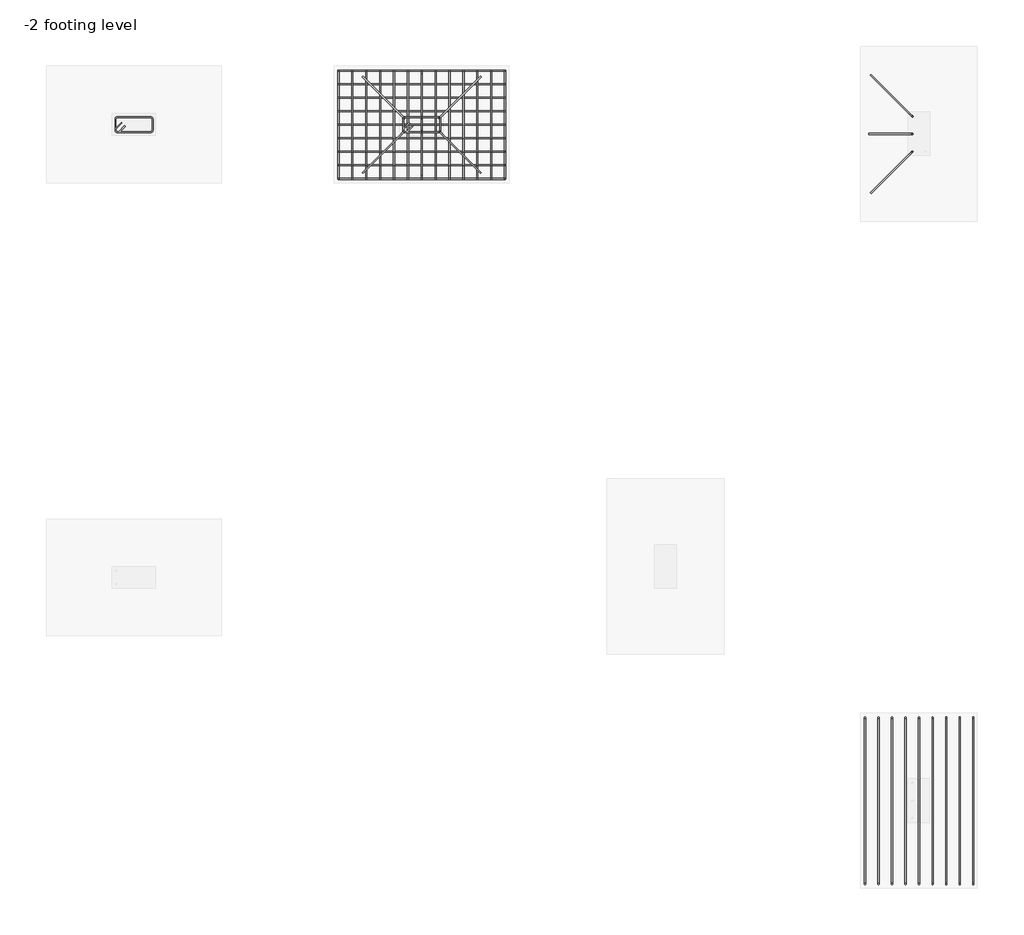
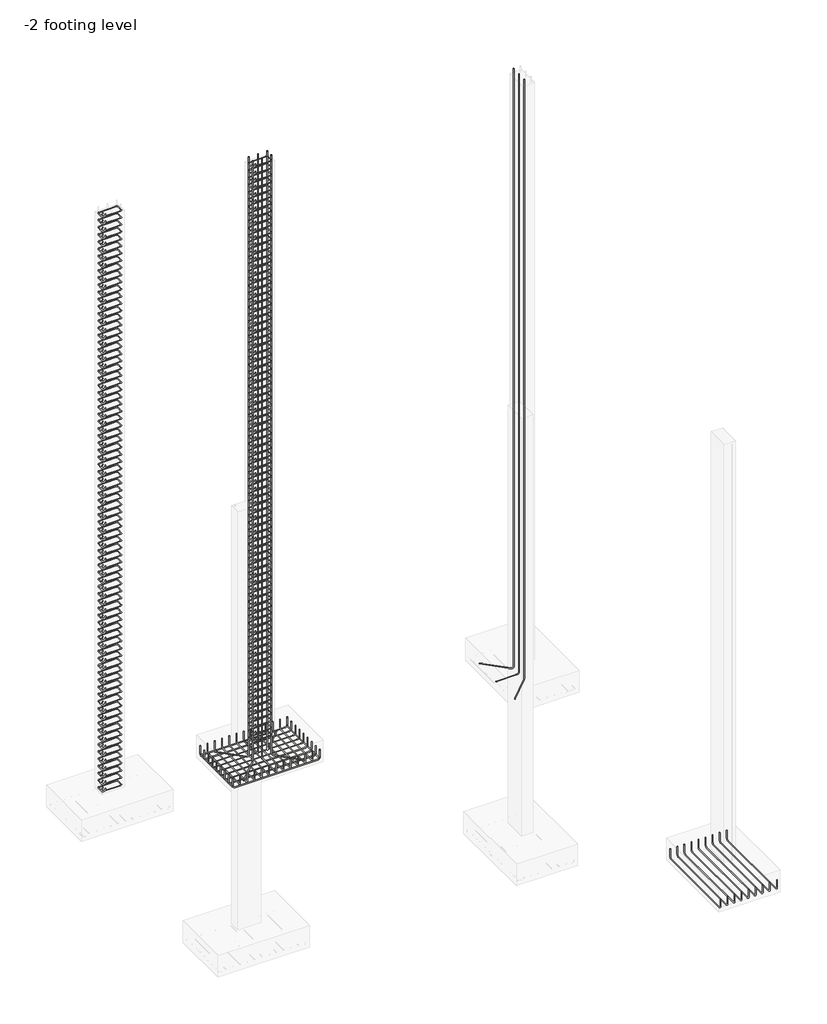
# One storey, part 3 of 9: 14 reinforcing bars.
"""IFC4 building model written with IfcOpenShell, lengths in millimetres."""

from ifc_helpers import new_model, si_unit, point, frame, origin, place, context, project, spatial, polyline, circle_curve, trimmed, segment, composite_curve, source, transform, mapped, element, save
from ifc_brep_helpers import swept_disk

model = new_model("IFC4")

# Units and contexts
model_context = context("Model", 3, world=origin())
ifc_project = project(units=[si_unit("LENGTHUNIT", "METRE", prefix="MILLI")], contexts=[model_context])

# Site, building, storey
site = spatial("IfcSite", under=ifc_project)
building = spatial("IfcBuilding", under=site)
storey = spatial("IfcBuildingStorey", under=building, Name="-2 footing level", Elevation=-1828.8)

# Reinforcing bars
placement = place(None, origin())
reinforcing_bar_shape = source(origin(), model_context, "Body", "SolidModel", [
    swept_disk(composite_curve([segment(polyline([(-4080.5198352, -1961.0445725, -2044.7), (-4080.5198352, -1961.0445725, -2197.1)]), True, "CONTINUOUS"), segment(trimmed(circle_curve(frame((-4124.9698352, -1961.0445725, -2197.1), z_axis=(0.0, 1.0, 0.0), x_axis=(44.44999999999936, 0.0, 0.0)), 44.45), [point((-4080.5198352, -1961.0445725, -2197.1))], [point((-4124.9698352, -1961.0445725, -2241.55))], True, "CARTESIAN"), True, "CONTINUOUS"), segment(polyline([(-4124.9698352, -1961.0445725, -2241.55), (-5775.9698352, -1961.0445725, -2241.55)]), True, "CONTINUOUS"), segment(trimmed(circle_curve(frame((-5775.9698352, -1961.0445725, -2197.1), z_axis=(0.0, 1.0, 0.0), x_axis=(0.0, 0.0, -44.45000000000027)), 44.45), [point((-5775.9698352, -1961.0445725, -2241.55))], [point((-5820.4198352, -1961.0445725, -2197.1))], True, "CARTESIAN"), True, "CONTINUOUS"), segment(polyline([(-5820.4198352, -1961.0445725, -2197.1), (-5820.4198352, -1961.0445725, -2044.7)]), True, "CONTINUOUS")], self_intersect=False), 6.35),
])
element("IfcReinforcingBar", 1, at=placement, inside=storey, context=model_context, shape_type="MappedRepresentation", body=[
    mapped(reinforcing_bar_shape, transform((0.0, 0.0, 0.0), x_axis=(1.0, 0.0, 0.0), y_axis=(0.0, 1.0, 0.0), z_axis=(0.0, 0.0, 1.0))),
    mapped(reinforcing_bar_shape, transform((0.0, -141.2875, 0.0), x_axis=(1.0, 0.0, 0.0), y_axis=(0.0, 1.0, 0.0), z_axis=(0.0, 0.0, 1.0))),
    mapped(reinforcing_bar_shape, transform((0.0, -282.575, 0.0), x_axis=(1.0, 0.0, 0.0), y_axis=(0.0, 1.0, 0.0), z_axis=(0.0, 0.0, 1.0))),
    mapped(reinforcing_bar_shape, transform((0.0, -423.8625, 0.0), x_axis=(1.0, 0.0, 0.0), y_axis=(0.0, 1.0, 0.0), z_axis=(0.0, 0.0, 1.0))),
    mapped(reinforcing_bar_shape, transform((0.0, -565.15, 0.0), x_axis=(1.0, 0.0, 0.0), y_axis=(0.0, 1.0, 0.0), z_axis=(0.0, 0.0, 1.0))),
    mapped(reinforcing_bar_shape, transform((0.0, -706.4375, 0.0), x_axis=(1.0, 0.0, 0.0), y_axis=(0.0, 1.0, 0.0), z_axis=(0.0, 0.0, 1.0))),
    mapped(reinforcing_bar_shape, transform((0.0, -847.725, 0.0), x_axis=(1.0, 0.0, 0.0), y_axis=(0.0, 1.0, 0.0), z_axis=(0.0, 0.0, 1.0))),
    mapped(reinforcing_bar_shape, transform((0.0, -989.0125, 0.0), x_axis=(1.0, 0.0, 0.0), y_axis=(0.0, 1.0, 0.0), z_axis=(0.0, 0.0, 1.0))),
    mapped(reinforcing_bar_shape, transform((0.0, -1130.3, 0.0), x_axis=(1.0, 0.0, 0.0), y_axis=(0.0, 1.0, 0.0), z_axis=(0.0, 0.0, 1.0))),
])
reinforcing_bar_2_shape = source(origin(), model_context, "Body", "SolidModel", [
    swept_disk(composite_curve([segment(polyline([(-5820.4198352, -1961.0445725, -2033.4041416), (-5820.4198352, -1961.0445725, -2185.8041416)]), True, "CONTINUOUS"), segment(trimmed(circle_curve(frame((-5820.4198352, -2005.4945725, -2185.8041416), z_axis=(-1.0, 0.0, 0.0), x_axis=(0.0, 44.450000000000045, 0.0)), 44.45), [point((-5820.4198352, -1961.0445725, -2185.8041416))], [point((-5820.4198352, -2005.4945725, -2230.2541416))], True, "CARTESIAN"), True, "CONTINUOUS"), segment(polyline([(-5820.4198352, -2005.4945725, -2230.2541416), (-5820.4198352, -3046.8945725, -2230.2541416)]), True, "CONTINUOUS"), segment(trimmed(circle_curve(frame((-5820.4198352, -3046.8945725, -2185.8041416), z_axis=(-1.0, 0.0, 0.0), x_axis=(0.0, 0.0, -44.44999999999982)), 44.45), [point((-5820.4198352, -3046.8945725, -2230.2541416))], [point((-5820.4198352, -3091.3445725, -2185.8041416))], True, "CARTESIAN"), True, "CONTINUOUS"), segment(polyline([(-5820.4198352, -3091.3445725, -2185.8041416), (-5820.4198352, -3091.3445725, -2033.4041416)]), True, "CONTINUOUS")], self_intersect=False), 6.35),
])
element("IfcReinforcingBar", 2, at=placement, inside=storey, context=model_context, shape_type="MappedRepresentation", body=[
    mapped(reinforcing_bar_2_shape, transform((0.0, 0.0, 0.0), x_axis=(1.0, 0.0, 0.0), y_axis=(0.0, 1.0, 0.0), z_axis=(0.0, 0.0, 1.0))),
    mapped(reinforcing_bar_2_shape, transform((144.9916667, 0.0, 0.0), x_axis=(1.0, 0.0, 0.0), y_axis=(0.0, 1.0, 0.0), z_axis=(0.0, 0.0, 1.0))),
    mapped(reinforcing_bar_2_shape, transform((289.9833333, 0.0, 0.0), x_axis=(1.0, 0.0, 0.0), y_axis=(0.0, 1.0, 0.0), z_axis=(0.0, 0.0, 1.0))),
    mapped(reinforcing_bar_2_shape, transform((434.975, 0.0, 0.0), x_axis=(1.0, 0.0, 0.0), y_axis=(0.0, 1.0, 0.0), z_axis=(0.0, 0.0, 1.0))),
    mapped(reinforcing_bar_2_shape, transform((579.9666667, 0.0, 0.0), x_axis=(1.0, 0.0, 0.0), y_axis=(0.0, 1.0, 0.0), z_axis=(0.0, 0.0, 1.0))),
    mapped(reinforcing_bar_2_shape, transform((724.9583333, 0.0, 0.0), x_axis=(1.0, 0.0, 0.0), y_axis=(0.0, 1.0, 0.0), z_axis=(0.0, 0.0, 1.0))),
    mapped(reinforcing_bar_2_shape, transform((869.95, 0.0, 0.0), x_axis=(1.0, 0.0, 0.0), y_axis=(0.0, 1.0, 0.0), z_axis=(0.0, 0.0, 1.0))),
    mapped(reinforcing_bar_2_shape, transform((1014.9416667, 0.0, 0.0), x_axis=(1.0, 0.0, 0.0), y_axis=(0.0, 1.0, 0.0), z_axis=(0.0, 0.0, 1.0))),
    mapped(reinforcing_bar_2_shape, transform((1159.9333333, 0.0, 0.0), x_axis=(1.0, 0.0, 0.0), y_axis=(0.0, 1.0, 0.0), z_axis=(0.0, 0.0, 1.0))),
    mapped(reinforcing_bar_2_shape, transform((1304.925, 0.0, 0.0), x_axis=(1.0, 0.0, 0.0), y_axis=(0.0, 1.0, 0.0), z_axis=(0.0, 0.0, 1.0))),
    mapped(reinforcing_bar_2_shape, transform((1449.9166667, 0.0, 0.0), x_axis=(1.0, 0.0, 0.0), y_axis=(0.0, 1.0, 0.0), z_axis=(0.0, 0.0, 1.0))),
    mapped(reinforcing_bar_2_shape, transform((1594.9083333, 0.0, 0.0), x_axis=(1.0, 0.0, 0.0), y_axis=(0.0, 1.0, 0.0), z_axis=(0.0, 0.0, 1.0))),
    mapped(reinforcing_bar_2_shape, transform((1739.9, 0.0, 0.0), x_axis=(1.0, 0.0, 0.0), y_axis=(0.0, 1.0, 0.0), z_axis=(0.0, 0.0, 1.0))),
])
reinforcing_bar_3_shape = source(origin(), model_context, "Body", "SolidModel", [
    swept_disk(composite_curve([segment(polyline([(-321.1911705, -8721.6294723, -2044.7), (-321.1911705, -8721.6294723, -2197.1)]), True, "CONTINUOUS"), segment(trimmed(circle_curve(frame((-321.1911705, -8766.0794723, -2197.1), z_axis=(-1.0, 0.0, 0.0), x_axis=(0.0, 44.45000000000073, 0.0)), 44.45), [point((-321.1911705, -8721.6294723, -2197.1))], [point((-321.1911705, -8766.0794723, -2241.55))], True, "CARTESIAN"), True, "CONTINUOUS"), segment(polyline([(-321.1911705, -8766.0794723, -2241.55), (-321.1911705, -10417.0794723, -2241.55)]), True, "CONTINUOUS"), segment(trimmed(circle_curve(frame((-321.1911705, -10417.0794723, -2197.1), z_axis=(-1.0, 0.0, 0.0), x_axis=(0.0, 0.0, -44.45000000000027)), 44.45), [point((-321.1911705, -10417.0794723, -2241.55))], [point((-321.1911705, -10461.5294723, -2197.1))], True, "CARTESIAN"), True, "CONTINUOUS"), segment(polyline([(-321.1911705, -10461.5294723, -2197.1), (-321.1911705, -10461.5294723, -2044.7)]), True, "CONTINUOUS")], self_intersect=False), 6.35),
])
element("IfcReinforcingBar", 3, at=placement, inside=storey, context=model_context, shape_type="MappedRepresentation", body=[
    mapped(reinforcing_bar_3_shape, transform((0.0, 0.0, 0.0), x_axis=(1.0, 0.0, 0.0), y_axis=(0.0, 1.0, 0.0), z_axis=(0.0, 0.0, 1.0))),
    mapped(reinforcing_bar_3_shape, transform((141.2875, 0.0, 0.0), x_axis=(1.0, 0.0, 0.0), y_axis=(0.0, 1.0, 0.0), z_axis=(0.0, 0.0, 1.0))),
    mapped(reinforcing_bar_3_shape, transform((282.575, 0.0, 0.0), x_axis=(1.0, 0.0, 0.0), y_axis=(0.0, 1.0, 0.0), z_axis=(0.0, 0.0, 1.0))),
    mapped(reinforcing_bar_3_shape, transform((423.8625, 0.0, 0.0), x_axis=(1.0, 0.0, 0.0), y_axis=(0.0, 1.0, 0.0), z_axis=(0.0, 0.0, 1.0))),
    mapped(reinforcing_bar_3_shape, transform((565.15, 0.0, 0.0), x_axis=(1.0, 0.0, 0.0), y_axis=(0.0, 1.0, 0.0), z_axis=(0.0, 0.0, 1.0))),
    mapped(reinforcing_bar_3_shape, transform((706.4375, 0.0, 0.0), x_axis=(1.0, 0.0, 0.0), y_axis=(0.0, 1.0, 0.0), z_axis=(0.0, 0.0, 1.0))),
    mapped(reinforcing_bar_3_shape, transform((847.725, 0.0, 0.0), x_axis=(1.0, 0.0, 0.0), y_axis=(0.0, 1.0, 0.0), z_axis=(0.0, 0.0, 1.0))),
    mapped(reinforcing_bar_3_shape, transform((989.0125, 0.0, 0.0), x_axis=(1.0, 0.0, 0.0), y_axis=(0.0, 1.0, 0.0), z_axis=(0.0, 0.0, 1.0))),
    mapped(reinforcing_bar_3_shape, transform((1130.3, 0.0, 0.0), x_axis=(1.0, 0.0, 0.0), y_axis=(0.0, 1.0, 0.0), z_axis=(0.0, 0.0, 1.0))),
])
element("IfcReinforcingBar", 4, at=placement, inside=storey, context=model_context, shape_type="SolidModel", body=[
    swept_disk(composite_curve([segment(polyline([(-259.3446547, -3240.9386149, -2212.9582082), (142.6779331, -2838.9160271, -2212.9582082)]), True, "CONTINUOUS"), segment(trimmed(circle_curve(frame((142.6779331, -2838.9160271, -2168.5082082), z_axis=(0.7071067811865501, -0.7071067811865449, 0.0), x_axis=(0.0, 0.0, -44.45000000000027)), 44.45), [point((142.6779331, -2838.9160271, -2212.9582082))], [point((174.1088295, -2807.4851307, -2168.5082082))], True, "CARTESIAN"), True, "CONTINUOUS"), segment(polyline([(174.1088295, -2807.4851307, -2168.5082082), (174.1088295, -2807.4851307, 10477.5)]), True, "CONTINUOUS")], self_intersect=False), 6.35),
])
element("IfcReinforcingBar", 5, at=placement, inside=storey, context=model_context, shape_type="SolidModel", body=[
    swept_disk(composite_curve([segment(polyline([(-259.3446547, -2005.7316465, -2212.9582082), (142.6779331, -2407.7542342, -2212.9582082)]), True, "CONTINUOUS"), segment(trimmed(circle_curve(frame((142.6779331, -2407.7542342, -2168.5082082), z_axis=(-0.7071067811865501, -0.7071067811865449, 0.0), x_axis=(0.0, 0.0, -44.45000000000027)), 44.45), [point((142.6779331, -2407.7542342, -2212.9582082))], [point((174.1088295, -2439.1851307, -2168.5082082))], True, "CARTESIAN"), True, "CONTINUOUS"), segment(polyline([(174.1088295, -2439.1851307, -2168.5082082), (174.1088295, -2439.1851307, 10477.5)]), True, "CONTINUOUS")], self_intersect=False), 6.35),
])
element("IfcReinforcingBar", 6, at=placement, inside=storey, context=model_context, shape_type="SolidModel", body=[
    swept_disk(composite_curve([segment(polyline([(-283.0911705, -2623.3351307, -2212.9582082), (129.6588295, -2623.3351307, -2212.9582082)]), True, "CONTINUOUS"), segment(trimmed(circle_curve(frame((129.6588295, -2623.3351307, -2168.5082082), z_axis=(0.0, -1.0, 0.0), x_axis=(0.0, 0.0, -44.45000000000027)), 44.45), [point((129.6588295, -2623.3351307, -2212.9582082))], [point((174.1088295, -2623.3351307, -2168.5082082))], True, "CARTESIAN"), True, "CONTINUOUS"), segment(polyline([(174.1088295, -2623.3351307, -2168.5082082), (174.1088295, -2623.3351307, 10477.5)]), True, "CONTINUOUS")], self_intersect=False), 6.35),
])
reinforcing_bar_4_shape = source(origin(), model_context, "Body", "SolidModel", [
    swept_disk(composite_curve([segment(polyline([(-8086.1371138, -2508.2533327, -1794.0734375), (-8143.0013108, -2565.1175298, -1794.0734375)]), True, "CONTINUOUS"), segment(trimmed(circle_curve(frame((-8126.1633306, -2581.95551, -1794.0734375), z_axis=(0.0, 0.0, 1.0), x_axis=(-16.837980199999947, 16.837980199999947, 0.0)), 23.8125), [point((-8143.0013108, -2565.1175298, -1794.0734375))], [point((-8126.1633306, -2605.76801, -1794.0734375))], True, "CARTESIAN"), True, "CONTINUOUS"), segment(polyline([(-8126.1633306, -2605.76801, -1794.0734375), (-7786.0414556, -2605.76801, -1794.0734375)]), True, "CONTINUOUS"), segment(trimmed(circle_curve(frame((-7786.0414556, -2581.95551, -1794.0734375), z_axis=(0.0, 0.0, 1.0), x_axis=(0.0, -23.8125, 0.0)), 23.8125), [point((-7786.0414556, -2605.76801, -1794.0734375))], [point((-7762.2289556, -2581.95551, -1794.0734375))], True, "CARTESIAN"), True, "CONTINUOUS"), segment(polyline([(-7762.2289556, -2581.95551, -1794.0734375), (-7762.2289556, -2470.433635, -1794.0734375)]), True, "CONTINUOUS"), segment(trimmed(circle_curve(frame((-7786.0342742, -2470.433635, -1794.658215), z_axis=(-0.024557586497356516, 0.0, 0.9996984169965585), x_axis=(23.805318600000646, 0.0, 0.5847774999999729)), 23.8125), [point((-7762.2289556, -2470.433635, -1794.0734375))], [point((-7786.0342742, -2446.621135, -1794.658215))], True, "CARTESIAN"), True, "CONTINUOUS"), segment(polyline([(-7786.0342742, -2446.621135, -1794.658215), (-8126.170512, -2446.621135, -1803.01366)]), True, "CONTINUOUS"), segment(trimmed(circle_curve(frame((-8126.170512, -2470.433635, -1803.01366), z_axis=(-0.024557586497356516, 0.0, 0.9996984169965585), x_axis=(0.0, 23.8125, 0.0)), 23.8125), [point((-8126.170512, -2446.621135, -1803.01366))], [point((-8149.9758306, -2470.433635, -1803.5984375))], True, "CARTESIAN"), True, "CONTINUOUS"), segment(polyline([(-8149.9758306, -2470.433635, -1803.5984375), (-8149.9758306, -2581.95551, -1803.5984375)]), True, "CONTINUOUS"), segment(trimmed(circle_curve(frame((-8126.1633306, -2581.95551, -1803.5984375), z_axis=(0.0, 0.0, 1.0), x_axis=(-23.8125, 0.0, 0.0)), 23.8125), [point((-8149.9758306, -2581.95551, -1803.5984375))], [point((-8109.3253504, -2598.7934902, -1803.5984375))], True, "CARTESIAN"), True, "CONTINUOUS"), segment(polyline([(-8109.3253504, -2598.7934902, -1803.5984375), (-8052.4611533, -2541.9292932, -1803.5984375)]), True, "CONTINUOUS")], self_intersect=False), 4.7625),
])
element("IfcReinforcingBar", 7, at=placement, inside=storey, context=model_context, shape_type="MappedRepresentation", body=[
    mapped(reinforcing_bar_4_shape, transform((0.0, 0.0, 0.0), x_axis=(1.0, 0.0, 0.0), y_axis=(0.0, 1.0, 0.0), z_axis=(0.0, 0.0, 1.0))),
    mapped(reinforcing_bar_4_shape, transform((0.0, 0.0, 151.9063867), x_axis=(1.0, 0.0, 0.0), y_axis=(0.0, 1.0, 0.0), z_axis=(0.0, 0.0, 1.0))),
    mapped(reinforcing_bar_4_shape, transform((0.0, 0.0, 303.8127734), x_axis=(1.0, 0.0, 0.0), y_axis=(0.0, 1.0, 0.0), z_axis=(0.0, 0.0, 1.0))),
    mapped(reinforcing_bar_4_shape, transform((0.0, 0.0, 455.7191602), x_axis=(1.0, 0.0, 0.0), y_axis=(0.0, 1.0, 0.0), z_axis=(0.0, 0.0, 1.0))),
    mapped(reinforcing_bar_4_shape, transform((0.0, 0.0, 607.6255469), x_axis=(1.0, 0.0, 0.0), y_axis=(0.0, 1.0, 0.0), z_axis=(0.0, 0.0, 1.0))),
    mapped(reinforcing_bar_4_shape, transform((0.0, 0.0, 759.5319336), x_axis=(1.0, 0.0, 0.0), y_axis=(0.0, 1.0, 0.0), z_axis=(0.0, 0.0, 1.0))),
    mapped(reinforcing_bar_4_shape, transform((0.0, 0.0, 911.4383203), x_axis=(1.0, 0.0, 0.0), y_axis=(0.0, 1.0, 0.0), z_axis=(0.0, 0.0, 1.0))),
    mapped(reinforcing_bar_4_shape, transform((0.0, 0.0, 1063.344707), x_axis=(1.0, 0.0, 0.0), y_axis=(0.0, 1.0, 0.0), z_axis=(0.0, 0.0, 1.0))),
    mapped(reinforcing_bar_4_shape, transform((0.0, 0.0, 1215.2510937), x_axis=(1.0, 0.0, 0.0), y_axis=(0.0, 1.0, 0.0), z_axis=(0.0, 0.0, 1.0))),
    mapped(reinforcing_bar_4_shape, transform((0.0, 0.0, 1367.1574805), x_axis=(1.0, 0.0, 0.0), y_axis=(0.0, 1.0, 0.0), z_axis=(0.0, 0.0, 1.0))),
    mapped(reinforcing_bar_4_shape, transform((0.0, 0.0, 1519.0638672), x_axis=(1.0, 0.0, 0.0), y_axis=(0.0, 1.0, 0.0), z_axis=(0.0, 0.0, 1.0))),
    mapped(reinforcing_bar_4_shape, transform((0.0, 0.0, 1670.9702539), x_axis=(1.0, 0.0, 0.0), y_axis=(0.0, 1.0, 0.0), z_axis=(0.0, 0.0, 1.0))),
    mapped(reinforcing_bar_4_shape, transform((0.0, 0.0, 1822.8766406), x_axis=(1.0, 0.0, 0.0), y_axis=(0.0, 1.0, 0.0), z_axis=(0.0, 0.0, 1.0))),
    mapped(reinforcing_bar_4_shape, transform((0.0, 0.0, 1974.7830273), x_axis=(1.0, 0.0, 0.0), y_axis=(0.0, 1.0, 0.0), z_axis=(0.0, 0.0, 1.0))),
    mapped(reinforcing_bar_4_shape, transform((0.0, 0.0, 2126.6894141), x_axis=(1.0, 0.0, 0.0), y_axis=(0.0, 1.0, 0.0), z_axis=(0.0, 0.0, 1.0))),
    mapped(reinforcing_bar_4_shape, transform((0.0, 0.0, 2278.5958008), x_axis=(1.0, 0.0, 0.0), y_axis=(0.0, 1.0, 0.0), z_axis=(0.0, 0.0, 1.0))),
    mapped(reinforcing_bar_4_shape, transform((0.0, 0.0, 2430.5021875), x_axis=(1.0, 0.0, 0.0), y_axis=(0.0, 1.0, 0.0), z_axis=(0.0, 0.0, 1.0))),
    mapped(reinforcing_bar_4_shape, transform((0.0, 0.0, 2582.4085742), x_axis=(1.0, 0.0, 0.0), y_axis=(0.0, 1.0, 0.0), z_axis=(0.0, 0.0, 1.0))),
    mapped(reinforcing_bar_4_shape, transform((0.0, 0.0, 2734.3149609), x_axis=(1.0, 0.0, 0.0), y_axis=(0.0, 1.0, 0.0), z_axis=(0.0, 0.0, 1.0))),
    mapped(reinforcing_bar_4_shape, transform((0.0, 0.0, 2886.2213477), x_axis=(1.0, 0.0, 0.0), y_axis=(0.0, 1.0, 0.0), z_axis=(0.0, 0.0, 1.0))),
    mapped(reinforcing_bar_4_shape, transform((0.0, 0.0, 3038.1277344), x_axis=(1.0, 0.0, 0.0), y_axis=(0.0, 1.0, 0.0), z_axis=(0.0, 0.0, 1.0))),
    mapped(reinforcing_bar_4_shape, transform((0.0, 0.0, 3190.0341211), x_axis=(1.0, 0.0, 0.0), y_axis=(0.0, 1.0, 0.0), z_axis=(0.0, 0.0, 1.0))),
    mapped(reinforcing_bar_4_shape, transform((0.0, 0.0, 3341.9405078), x_axis=(1.0, 0.0, 0.0), y_axis=(0.0, 1.0, 0.0), z_axis=(0.0, 0.0, 1.0))),
    mapped(reinforcing_bar_4_shape, transform((0.0, 0.0, 3493.8468945), x_axis=(1.0, 0.0, 0.0), y_axis=(0.0, 1.0, 0.0), z_axis=(0.0, 0.0, 1.0))),
    mapped(reinforcing_bar_4_shape, transform((0.0, 0.0, 3645.7532812), x_axis=(1.0, 0.0, 0.0), y_axis=(0.0, 1.0, 0.0), z_axis=(0.0, 0.0, 1.0))),
    mapped(reinforcing_bar_4_shape, transform((0.0, 0.0, 3797.659668), x_axis=(1.0, 0.0, 0.0), y_axis=(0.0, 1.0, 0.0), z_axis=(0.0, 0.0, 1.0))),
    mapped(reinforcing_bar_4_shape, transform((0.0, 0.0, 3949.5660547), x_axis=(1.0, 0.0, 0.0), y_axis=(0.0, 1.0, 0.0), z_axis=(0.0, 0.0, 1.0))),
    mapped(reinforcing_bar_4_shape, transform((0.0, 0.0, 4101.4724414), x_axis=(1.0, 0.0, 0.0), y_axis=(0.0, 1.0, 0.0), z_axis=(0.0, 0.0, 1.0))),
    mapped(reinforcing_bar_4_shape, transform((0.0, 0.0, 4253.3788281), x_axis=(1.0, 0.0, 0.0), y_axis=(0.0, 1.0, 0.0), z_axis=(0.0, 0.0, 1.0))),
    mapped(reinforcing_bar_4_shape, transform((0.0, 0.0, 4405.2852148), x_axis=(1.0, 0.0, 0.0), y_axis=(0.0, 1.0, 0.0), z_axis=(0.0, 0.0, 1.0))),
    mapped(reinforcing_bar_4_shape, transform((0.0, 0.0, 4557.1916016), x_axis=(1.0, 0.0, 0.0), y_axis=(0.0, 1.0, 0.0), z_axis=(0.0, 0.0, 1.0))),
    mapped(reinforcing_bar_4_shape, transform((0.0, 0.0, 4709.0979883), x_axis=(1.0, 0.0, 0.0), y_axis=(0.0, 1.0, 0.0), z_axis=(0.0, 0.0, 1.0))),
    mapped(reinforcing_bar_4_shape, transform((0.0, 0.0, 4861.004375), x_axis=(1.0, 0.0, 0.0), y_axis=(0.0, 1.0, 0.0), z_axis=(0.0, 0.0, 1.0))),
    mapped(reinforcing_bar_4_shape, transform((0.0, 0.0, 5012.9107617), x_axis=(1.0, 0.0, 0.0), y_axis=(0.0, 1.0, 0.0), z_axis=(0.0, 0.0, 1.0))),
    mapped(reinforcing_bar_4_shape, transform((0.0, 0.0, 5164.8171484), x_axis=(1.0, 0.0, 0.0), y_axis=(0.0, 1.0, 0.0), z_axis=(0.0, 0.0, 1.0))),
    mapped(reinforcing_bar_4_shape, transform((0.0, 0.0, 5316.7235352), x_axis=(1.0, 0.0, 0.0), y_axis=(0.0, 1.0, 0.0), z_axis=(0.0, 0.0, 1.0))),
    mapped(reinforcing_bar_4_shape, transform((0.0, 0.0, 5468.6299219), x_axis=(1.0, 0.0, 0.0), y_axis=(0.0, 1.0, 0.0), z_axis=(0.0, 0.0, 1.0))),
    mapped(reinforcing_bar_4_shape, transform((0.0, 0.0, 5620.5363086), x_axis=(1.0, 0.0, 0.0), y_axis=(0.0, 1.0, 0.0), z_axis=(0.0, 0.0, 1.0))),
    mapped(reinforcing_bar_4_shape, transform((0.0, 0.0, 5772.4426953), x_axis=(1.0, 0.0, 0.0), y_axis=(0.0, 1.0, 0.0), z_axis=(0.0, 0.0, 1.0))),
    mapped(reinforcing_bar_4_shape, transform((0.0, 0.0, 5924.349082), x_axis=(1.0, 0.0, 0.0), y_axis=(0.0, 1.0, 0.0), z_axis=(0.0, 0.0, 1.0))),
    mapped(reinforcing_bar_4_shape, transform((0.0, 0.0, 6076.2554687), x_axis=(1.0, 0.0, 0.0), y_axis=(0.0, 1.0, 0.0), z_axis=(0.0, 0.0, 1.0))),
    mapped(reinforcing_bar_4_shape, transform((0.0, 0.0, 6228.1618555), x_axis=(1.0, 0.0, 0.0), y_axis=(0.0, 1.0, 0.0), z_axis=(0.0, 0.0, 1.0))),
    mapped(reinforcing_bar_4_shape, transform((0.0, 0.0, 6380.0682422), x_axis=(1.0, 0.0, 0.0), y_axis=(0.0, 1.0, 0.0), z_axis=(0.0, 0.0, 1.0))),
    mapped(reinforcing_bar_4_shape, transform((0.0, 0.0, 6531.9746289), x_axis=(1.0, 0.0, 0.0), y_axis=(0.0, 1.0, 0.0), z_axis=(0.0, 0.0, 1.0))),
    mapped(reinforcing_bar_4_shape, transform((0.0, 0.0, 6683.8810156), x_axis=(1.0, 0.0, 0.0), y_axis=(0.0, 1.0, 0.0), z_axis=(0.0, 0.0, 1.0))),
    mapped(reinforcing_bar_4_shape, transform((0.0, 0.0, 6835.7874023), x_axis=(1.0, 0.0, 0.0), y_axis=(0.0, 1.0, 0.0), z_axis=(0.0, 0.0, 1.0))),
    mapped(reinforcing_bar_4_shape, transform((0.0, 0.0, 6987.6937891), x_axis=(1.0, 0.0, 0.0), y_axis=(0.0, 1.0, 0.0), z_axis=(0.0, 0.0, 1.0))),
    mapped(reinforcing_bar_4_shape, transform((0.0, 0.0, 7139.6001758), x_axis=(1.0, 0.0, 0.0), y_axis=(0.0, 1.0, 0.0), z_axis=(0.0, 0.0, 1.0))),
    mapped(reinforcing_bar_4_shape, transform((0.0, 0.0, 7291.5065625), x_axis=(1.0, 0.0, 0.0), y_axis=(0.0, 1.0, 0.0), z_axis=(0.0, 0.0, 1.0))),
    mapped(reinforcing_bar_4_shape, transform((0.0, 0.0, 7443.4129492), x_axis=(1.0, 0.0, 0.0), y_axis=(0.0, 1.0, 0.0), z_axis=(0.0, 0.0, 1.0))),
    mapped(reinforcing_bar_4_shape, transform((0.0, 0.0, 7595.3193359), x_axis=(1.0, 0.0, 0.0), y_axis=(0.0, 1.0, 0.0), z_axis=(0.0, 0.0, 1.0))),
    mapped(reinforcing_bar_4_shape, transform((0.0, 0.0, 7747.2257227), x_axis=(1.0, 0.0, 0.0), y_axis=(0.0, 1.0, 0.0), z_axis=(0.0, 0.0, 1.0))),
    mapped(reinforcing_bar_4_shape, transform((0.0, 0.0, 7899.1321094), x_axis=(1.0, 0.0, 0.0), y_axis=(0.0, 1.0, 0.0), z_axis=(0.0, 0.0, 1.0))),
    mapped(reinforcing_bar_4_shape, transform((0.0, 0.0, 8051.0384961), x_axis=(1.0, 0.0, 0.0), y_axis=(0.0, 1.0, 0.0), z_axis=(0.0, 0.0, 1.0))),
    mapped(reinforcing_bar_4_shape, transform((0.0, 0.0, 8202.9448828), x_axis=(1.0, 0.0, 0.0), y_axis=(0.0, 1.0, 0.0), z_axis=(0.0, 0.0, 1.0))),
    mapped(reinforcing_bar_4_shape, transform((0.0, 0.0, 8354.8512695), x_axis=(1.0, 0.0, 0.0), y_axis=(0.0, 1.0, 0.0), z_axis=(0.0, 0.0, 1.0))),
    mapped(reinforcing_bar_4_shape, transform((0.0, 0.0, 8506.7576562), x_axis=(1.0, 0.0, 0.0), y_axis=(0.0, 1.0, 0.0), z_axis=(0.0, 0.0, 1.0))),
    mapped(reinforcing_bar_4_shape, transform((0.0, 0.0, 8658.664043), x_axis=(1.0, 0.0, 0.0), y_axis=(0.0, 1.0, 0.0), z_axis=(0.0, 0.0, 1.0))),
    mapped(reinforcing_bar_4_shape, transform((0.0, 0.0, 8810.5704297), x_axis=(1.0, 0.0, 0.0), y_axis=(0.0, 1.0, 0.0), z_axis=(0.0, 0.0, 1.0))),
    mapped(reinforcing_bar_4_shape, transform((0.0, 0.0, 8962.4768164), x_axis=(1.0, 0.0, 0.0), y_axis=(0.0, 1.0, 0.0), z_axis=(0.0, 0.0, 1.0))),
    mapped(reinforcing_bar_4_shape, transform((0.0, 0.0, 9114.3832031), x_axis=(1.0, 0.0, 0.0), y_axis=(0.0, 1.0, 0.0), z_axis=(0.0, 0.0, 1.0))),
    mapped(reinforcing_bar_4_shape, transform((0.0, 0.0, 9266.2895898), x_axis=(1.0, 0.0, 0.0), y_axis=(0.0, 1.0, 0.0), z_axis=(0.0, 0.0, 1.0))),
    mapped(reinforcing_bar_4_shape, transform((0.0, 0.0, 9418.1959766), x_axis=(1.0, 0.0, 0.0), y_axis=(0.0, 1.0, 0.0), z_axis=(0.0, 0.0, 1.0))),
    mapped(reinforcing_bar_4_shape, transform((0.0, 0.0, 9570.1023633), x_axis=(1.0, 0.0, 0.0), y_axis=(0.0, 1.0, 0.0), z_axis=(0.0, 0.0, 1.0))),
    mapped(reinforcing_bar_4_shape, transform((0.0, 0.0, 9722.00875), x_axis=(1.0, 0.0, 0.0), y_axis=(0.0, 1.0, 0.0), z_axis=(0.0, 0.0, 1.0))),
    mapped(reinforcing_bar_4_shape, transform((0.0, 0.0, 9873.9151367), x_axis=(1.0, 0.0, 0.0), y_axis=(0.0, 1.0, 0.0), z_axis=(0.0, 0.0, 1.0))),
    mapped(reinforcing_bar_4_shape, transform((0.0, 0.0, 10025.8215234), x_axis=(1.0, 0.0, 0.0), y_axis=(0.0, 1.0, 0.0), z_axis=(0.0, 0.0, 1.0))),
    mapped(reinforcing_bar_4_shape, transform((0.0, 0.0, 10177.7279102), x_axis=(1.0, 0.0, 0.0), y_axis=(0.0, 1.0, 0.0), z_axis=(0.0, 0.0, 1.0))),
    mapped(reinforcing_bar_4_shape, transform((0.0, 0.0, 10329.6342969), x_axis=(1.0, 0.0, 0.0), y_axis=(0.0, 1.0, 0.0), z_axis=(0.0, 0.0, 1.0))),
    mapped(reinforcing_bar_4_shape, transform((0.0, 0.0, 10481.5406836), x_axis=(1.0, 0.0, 0.0), y_axis=(0.0, 1.0, 0.0), z_axis=(0.0, 0.0, 1.0))),
    mapped(reinforcing_bar_4_shape, transform((0.0, 0.0, 10633.4470703), x_axis=(1.0, 0.0, 0.0), y_axis=(0.0, 1.0, 0.0), z_axis=(0.0, 0.0, 1.0))),
    mapped(reinforcing_bar_4_shape, transform((0.0, 0.0, 10785.353457), x_axis=(1.0, 0.0, 0.0), y_axis=(0.0, 1.0, 0.0), z_axis=(0.0, 0.0, 1.0))),
    mapped(reinforcing_bar_4_shape, transform((0.0, 0.0, 10937.2598437), x_axis=(1.0, 0.0, 0.0), y_axis=(0.0, 1.0, 0.0), z_axis=(0.0, 0.0, 1.0))),
    mapped(reinforcing_bar_4_shape, transform((0.0, 0.0, 11089.1662305), x_axis=(1.0, 0.0, 0.0), y_axis=(0.0, 1.0, 0.0), z_axis=(0.0, 0.0, 1.0))),
    mapped(reinforcing_bar_4_shape, transform((0.0, 0.0, 11241.0726172), x_axis=(1.0, 0.0, 0.0), y_axis=(0.0, 1.0, 0.0), z_axis=(0.0, 0.0, 1.0))),
    mapped(reinforcing_bar_4_shape, transform((0.0, 0.0, 11392.9790039), x_axis=(1.0, 0.0, 0.0), y_axis=(0.0, 1.0, 0.0), z_axis=(0.0, 0.0, 1.0))),
    mapped(reinforcing_bar_4_shape, transform((0.0, 0.0, 11544.8853906), x_axis=(1.0, 0.0, 0.0), y_axis=(0.0, 1.0, 0.0), z_axis=(0.0, 0.0, 1.0))),
    mapped(reinforcing_bar_4_shape, transform((0.0, 0.0, 11696.7917773), x_axis=(1.0, 0.0, 0.0), y_axis=(0.0, 1.0, 0.0), z_axis=(0.0, 0.0, 1.0))),
    mapped(reinforcing_bar_4_shape, transform((0.0, 0.0, 11848.6981641), x_axis=(1.0, 0.0, 0.0), y_axis=(0.0, 1.0, 0.0), z_axis=(0.0, 0.0, 1.0))),
    mapped(reinforcing_bar_4_shape, transform((0.0, 0.0, 12000.6045508), x_axis=(1.0, 0.0, 0.0), y_axis=(0.0, 1.0, 0.0), z_axis=(0.0, 0.0, 1.0))),
    mapped(reinforcing_bar_4_shape, transform((0.0, 0.0, 12152.5109375), x_axis=(1.0, 0.0, 0.0), y_axis=(0.0, 1.0, 0.0), z_axis=(0.0, 0.0, 1.0))),
])
element("IfcReinforcingBar", 8, at=placement, inside=storey, context=model_context, shape_type="SolidModel", body=[
    swept_disk(composite_curve([segment(polyline([(-5568.6755659, -2022.8910883, -2212.9582082), (-5166.6529781, -2424.9136761, -2212.9582082)]), True, "CONTINUOUS"), segment(trimmed(circle_curve(frame((-5166.6529781, -2424.9136761, -2168.5082082), z_axis=(-0.7071067811865455, -0.7071067811865496, 0.0), x_axis=(0.0, 0.0, -44.45000000000027)), 44.45), [point((-5166.6529781, -2424.9136761, -2212.9582082))], [point((-5135.2220817, -2456.3445725, -2168.5082082))], True, "CARTESIAN"), True, "CONTINUOUS"), segment(polyline([(-5135.2220817, -2456.3445725, -2168.5082082), (-5135.2220817, -2456.3445725, 10477.5)]), True, "CONTINUOUS")], self_intersect=False), 6.35),
])
element("IfcReinforcingBar", 9, at=placement, inside=storey, context=model_context, shape_type="SolidModel", body=[
    swept_disk(composite_curve([segment(polyline([(-5568.6755659, -3029.4980567, -2212.9582082), (-5166.6529781, -2627.4754689, -2212.9582082)]), True, "CONTINUOUS"), segment(trimmed(circle_curve(frame((-5166.6529781, -2627.4754689, -2168.5082082), z_axis=(0.707106781186541, -0.707106781186554, 0.0), x_axis=(0.0, 0.0, -44.45000000000027)), 44.45), [point((-5166.6529781, -2627.4754689, -2212.9582082))], [point((-5135.2220817, -2596.0445725, -2168.5082082))], True, "CARTESIAN"), True, "CONTINUOUS"), segment(polyline([(-5135.2220817, -2596.0445725, -2168.5082082), (-5135.2220817, -2596.0445725, 10477.5)]), True, "CONTINUOUS")], self_intersect=False), 6.35),
])
element("IfcReinforcingBar", 10, at=placement, inside=storey, context=model_context, shape_type="SolidModel", body=[
    swept_disk(composite_curve([segment(polyline([(-4333.4685975, -2022.8910883, -2212.9582082), (-4735.4911853, -2424.9136761, -2212.9582082)]), True, "CONTINUOUS"), segment(trimmed(circle_curve(frame((-4735.4911853, -2424.9136761, -2168.5082082), z_axis=(-0.7071067811865444, 0.7071067811865507, 0.0), x_axis=(0.0, 0.0, -44.45000000000027)), 44.45), [point((-4735.4911853, -2424.9136761, -2212.9582082))], [point((-4766.9220817, -2456.3445725, -2168.5082082))], True, "CARTESIAN"), True, "CONTINUOUS"), segment(polyline([(-4766.9220817, -2456.3445725, -2168.5082082), (-4766.9220817, -2456.3445725, 10477.5)]), True, "CONTINUOUS")], self_intersect=False), 6.35),
])
element("IfcReinforcingBar", 11, at=placement, inside=storey, context=model_context, shape_type="SolidModel", body=[
    swept_disk(composite_curve([segment(polyline([(-4333.4685975, -3029.4980567, -2212.9582082), (-4735.4911853, -2627.4754689, -2212.9582082)]), True, "CONTINUOUS"), segment(trimmed(circle_curve(frame((-4735.4911853, -2627.4754689, -2168.5082082), z_axis=(0.7071067811865421, 0.7071067811865529, 0.0), x_axis=(0.0, 0.0, -44.45000000000027)), 44.45), [point((-4735.4911853, -2627.4754689, -2212.9582082))], [point((-4766.9220817, -2596.0445725, -2168.5082082))], True, "CARTESIAN"), True, "CONTINUOUS"), segment(polyline([(-4766.9220817, -2596.0445725, -2168.5082082), (-4766.9220817, -2596.0445725, 10477.5)]), True, "CONTINUOUS")], self_intersect=False), 6.35),
])
element("IfcReinforcingBar", 12, at=placement, inside=storey, context=model_context, shape_type="SolidModel", body=[
    swept_disk(composite_curve([segment(polyline([(-4951.0720817, -1999.1445725, -2212.9582082), (-4951.0720817, -2413.283635, -2212.9582082)]), True, "CONTINUOUS"), segment(trimmed(circle_curve(frame((-4951.0720817, -2413.283635, -2168.5082082), z_axis=(-1.0, 0.0, 0.0), x_axis=(0.0, 0.0, -44.45000000000027)), 44.45), [point((-4951.0720817, -2413.283635, -2212.9582082))], [point((-4951.0720817, -2457.733635, -2168.5082082))], True, "CARTESIAN"), True, "CONTINUOUS"), segment(polyline([(-4951.0720817, -2457.733635, -2168.5082082), (-4951.0720817, -2457.733635, 10477.5)]), True, "CONTINUOUS")], self_intersect=False), 6.35),
])
element("IfcReinforcingBar", 13, at=placement, inside=storey, context=model_context, shape_type="SolidModel", body=[
    swept_disk(composite_curve([segment(polyline([(-4951.0720817, -3053.2445725, -2212.9582082), (-4951.0720817, -2639.10551, -2212.9582082)]), True, "CONTINUOUS"), segment(trimmed(circle_curve(frame((-4951.0720817, -2639.10551, -2168.5082082), z_axis=(1.0, 0.0, 0.0), x_axis=(0.0, 0.0, -44.45000000000027)), 44.45), [point((-4951.0720817, -2639.10551, -2212.9582082))], [point((-4951.0720817, -2594.65551, -2168.5082082))], True, "CARTESIAN"), True, "CONTINUOUS"), segment(polyline([(-4951.0720817, -2594.65551, -2168.5082082), (-4951.0720817, -2594.65551, 10477.5)]), True, "CONTINUOUS")], self_intersect=False), 6.35),
])
reinforcing_bar_5_shape = source(origin(), model_context, "Body", "SolidModel", [
    swept_disk(composite_curve([segment(polyline([(-5081.1068024, -2508.2533327, -1794.0734375), (-5137.9709994, -2565.1175298, -1794.0734375)]), True, "CONTINUOUS"), segment(trimmed(circle_curve(frame((-5121.1330192, -2581.95551, -1794.0734375), z_axis=(0.0, 0.0, 1.0), x_axis=(-16.837980200000857, 16.837980199999947, 0.0)), 23.8125), [point((-5137.9709994, -2565.1175298, -1794.0734375))], [point((-5121.1330192, -2605.76801, -1794.0734375))], True, "CARTESIAN"), True, "CONTINUOUS"), segment(polyline([(-5121.1330192, -2605.76801, -1794.0734375), (-4781.0111442, -2605.76801, -1794.0734375)]), True, "CONTINUOUS"), segment(trimmed(circle_curve(frame((-4781.0111442, -2581.95551, -1794.0734375), z_axis=(0.0, 0.0, 1.0), x_axis=(0.0, -23.8125, 0.0)), 23.8125), [point((-4781.0111442, -2605.76801, -1794.0734375))], [point((-4757.1986442, -2581.95551, -1794.0734375))], True, "CARTESIAN"), True, "CONTINUOUS"), segment(polyline([(-4757.1986442, -2581.95551, -1794.0734375), (-4757.1986442, -2470.433635, -1794.0734375)]), True, "CONTINUOUS"), segment(trimmed(circle_curve(frame((-4781.0039627, -2470.433635, -1794.658215), z_axis=(-0.024557586497356516, 0.0, 0.9996984169965585), x_axis=(23.805318499999885, 0.0, 0.5847774999999729)), 23.8125), [point((-4757.1986442, -2470.433635, -1794.0734375))], [point((-4781.0039627, -2446.621135, -1794.658215))], True, "CARTESIAN"), True, "CONTINUOUS"), segment(polyline([(-4781.0039627, -2446.621135, -1794.658215), (-5121.1402006, -2446.621135, -1803.01366)]), True, "CONTINUOUS"), segment(trimmed(circle_curve(frame((-5121.1402006, -2470.433635, -1803.01366), z_axis=(-0.024557586497356516, 0.0, 0.9996984169965585), x_axis=(0.0, 23.8125, 0.0)), 23.8125), [point((-5121.1402006, -2446.621135, -1803.01366))], [point((-5144.9455192, -2470.433635, -1803.5984375))], True, "CARTESIAN"), True, "CONTINUOUS"), segment(polyline([(-5144.9455192, -2470.433635, -1803.5984375), (-5144.9455192, -2581.95551, -1803.5984375)]), True, "CONTINUOUS"), segment(trimmed(circle_curve(frame((-5121.1330192, -2581.95551, -1803.5984375), z_axis=(0.0, 0.0, 1.0), x_axis=(-23.8125, 0.0, 0.0)), 23.8125), [point((-5144.9455192, -2581.95551, -1803.5984375))], [point((-5104.295039, -2598.7934902, -1803.5984375))], True, "CARTESIAN"), True, "CONTINUOUS"), segment(polyline([(-5104.295039, -2598.7934902, -1803.5984375), (-5047.4308419, -2541.9292932, -1803.5984375)]), True, "CONTINUOUS")], self_intersect=False), 4.7625),
])
element("IfcReinforcingBar", 14, at=placement, inside=storey, context=model_context, shape_type="MappedRepresentation", body=[
    mapped(reinforcing_bar_5_shape, transform((0.0, 0.0, 0.0), x_axis=(1.0, 0.0, 0.0), y_axis=(0.0, 1.0, 0.0), z_axis=(0.0, 0.0, 1.0))),
    mapped(reinforcing_bar_5_shape, transform((0.0, 0.0, 151.9063867), x_axis=(1.0, 0.0, 0.0), y_axis=(0.0, 1.0, 0.0), z_axis=(0.0, 0.0, 1.0))),
    mapped(reinforcing_bar_5_shape, transform((0.0, 0.0, 303.8127734), x_axis=(1.0, 0.0, 0.0), y_axis=(0.0, 1.0, 0.0), z_axis=(0.0, 0.0, 1.0))),
    mapped(reinforcing_bar_5_shape, transform((0.0, 0.0, 455.7191602), x_axis=(1.0, 0.0, 0.0), y_axis=(0.0, 1.0, 0.0), z_axis=(0.0, 0.0, 1.0))),
    mapped(reinforcing_bar_5_shape, transform((0.0, 0.0, 607.6255469), x_axis=(1.0, 0.0, 0.0), y_axis=(0.0, 1.0, 0.0), z_axis=(0.0, 0.0, 1.0))),
    mapped(reinforcing_bar_5_shape, transform((0.0, 0.0, 759.5319336), x_axis=(1.0, 0.0, 0.0), y_axis=(0.0, 1.0, 0.0), z_axis=(0.0, 0.0, 1.0))),
    mapped(reinforcing_bar_5_shape, transform((0.0, 0.0, 911.4383203), x_axis=(1.0, 0.0, 0.0), y_axis=(0.0, 1.0, 0.0), z_axis=(0.0, 0.0, 1.0))),
    mapped(reinforcing_bar_5_shape, transform((0.0, 0.0, 1063.344707), x_axis=(1.0, 0.0, 0.0), y_axis=(0.0, 1.0, 0.0), z_axis=(0.0, 0.0, 1.0))),
    mapped(reinforcing_bar_5_shape, transform((0.0, 0.0, 1215.2510937), x_axis=(1.0, 0.0, 0.0), y_axis=(0.0, 1.0, 0.0), z_axis=(0.0, 0.0, 1.0))),
    mapped(reinforcing_bar_5_shape, transform((0.0, 0.0, 1367.1574805), x_axis=(1.0, 0.0, 0.0), y_axis=(0.0, 1.0, 0.0), z_axis=(0.0, 0.0, 1.0))),
    mapped(reinforcing_bar_5_shape, transform((0.0, 0.0, 1519.0638672), x_axis=(1.0, 0.0, 0.0), y_axis=(0.0, 1.0, 0.0), z_axis=(0.0, 0.0, 1.0))),
    mapped(reinforcing_bar_5_shape, transform((0.0, 0.0, 1670.9702539), x_axis=(1.0, 0.0, 0.0), y_axis=(0.0, 1.0, 0.0), z_axis=(0.0, 0.0, 1.0))),
    mapped(reinforcing_bar_5_shape, transform((0.0, 0.0, 1822.8766406), x_axis=(1.0, 0.0, 0.0), y_axis=(0.0, 1.0, 0.0), z_axis=(0.0, 0.0, 1.0))),
    mapped(reinforcing_bar_5_shape, transform((0.0, 0.0, 1974.7830273), x_axis=(1.0, 0.0, 0.0), y_axis=(0.0, 1.0, 0.0), z_axis=(0.0, 0.0, 1.0))),
    mapped(reinforcing_bar_5_shape, transform((0.0, 0.0, 2126.6894141), x_axis=(1.0, 0.0, 0.0), y_axis=(0.0, 1.0, 0.0), z_axis=(0.0, 0.0, 1.0))),
    mapped(reinforcing_bar_5_shape, transform((0.0, 0.0, 2278.5958008), x_axis=(1.0, 0.0, 0.0), y_axis=(0.0, 1.0, 0.0), z_axis=(0.0, 0.0, 1.0))),
    mapped(reinforcing_bar_5_shape, transform((0.0, 0.0, 2430.5021875), x_axis=(1.0, 0.0, 0.0), y_axis=(0.0, 1.0, 0.0), z_axis=(0.0, 0.0, 1.0))),
    mapped(reinforcing_bar_5_shape, transform((0.0, 0.0, 2582.4085742), x_axis=(1.0, 0.0, 0.0), y_axis=(0.0, 1.0, 0.0), z_axis=(0.0, 0.0, 1.0))),
    mapped(reinforcing_bar_5_shape, transform((0.0, 0.0, 2734.3149609), x_axis=(1.0, 0.0, 0.0), y_axis=(0.0, 1.0, 0.0), z_axis=(0.0, 0.0, 1.0))),
    mapped(reinforcing_bar_5_shape, transform((0.0, 0.0, 2886.2213477), x_axis=(1.0, 0.0, 0.0), y_axis=(0.0, 1.0, 0.0), z_axis=(0.0, 0.0, 1.0))),
    mapped(reinforcing_bar_5_shape, transform((0.0, 0.0, 3038.1277344), x_axis=(1.0, 0.0, 0.0), y_axis=(0.0, 1.0, 0.0), z_axis=(0.0, 0.0, 1.0))),
    mapped(reinforcing_bar_5_shape, transform((0.0, 0.0, 3190.0341211), x_axis=(1.0, 0.0, 0.0), y_axis=(0.0, 1.0, 0.0), z_axis=(0.0, 0.0, 1.0))),
    mapped(reinforcing_bar_5_shape, transform((0.0, 0.0, 3341.9405078), x_axis=(1.0, 0.0, 0.0), y_axis=(0.0, 1.0, 0.0), z_axis=(0.0, 0.0, 1.0))),
    mapped(reinforcing_bar_5_shape, transform((0.0, 0.0, 3493.8468945), x_axis=(1.0, 0.0, 0.0), y_axis=(0.0, 1.0, 0.0), z_axis=(0.0, 0.0, 1.0))),
    mapped(reinforcing_bar_5_shape, transform((0.0, 0.0, 3645.7532812), x_axis=(1.0, 0.0, 0.0), y_axis=(0.0, 1.0, 0.0), z_axis=(0.0, 0.0, 1.0))),
    mapped(reinforcing_bar_5_shape, transform((0.0, 0.0, 3797.659668), x_axis=(1.0, 0.0, 0.0), y_axis=(0.0, 1.0, 0.0), z_axis=(0.0, 0.0, 1.0))),
    mapped(reinforcing_bar_5_shape, transform((0.0, 0.0, 3949.5660547), x_axis=(1.0, 0.0, 0.0), y_axis=(0.0, 1.0, 0.0), z_axis=(0.0, 0.0, 1.0))),
    mapped(reinforcing_bar_5_shape, transform((0.0, 0.0, 4101.4724414), x_axis=(1.0, 0.0, 0.0), y_axis=(0.0, 1.0, 0.0), z_axis=(0.0, 0.0, 1.0))),
    mapped(reinforcing_bar_5_shape, transform((0.0, 0.0, 4253.3788281), x_axis=(1.0, 0.0, 0.0), y_axis=(0.0, 1.0, 0.0), z_axis=(0.0, 0.0, 1.0))),
    mapped(reinforcing_bar_5_shape, transform((0.0, 0.0, 4405.2852148), x_axis=(1.0, 0.0, 0.0), y_axis=(0.0, 1.0, 0.0), z_axis=(0.0, 0.0, 1.0))),
    mapped(reinforcing_bar_5_shape, transform((0.0, 0.0, 4557.1916016), x_axis=(1.0, 0.0, 0.0), y_axis=(0.0, 1.0, 0.0), z_axis=(0.0, 0.0, 1.0))),
    mapped(reinforcing_bar_5_shape, transform((0.0, 0.0, 4709.0979883), x_axis=(1.0, 0.0, 0.0), y_axis=(0.0, 1.0, 0.0), z_axis=(0.0, 0.0, 1.0))),
    mapped(reinforcing_bar_5_shape, transform((0.0, 0.0, 4861.004375), x_axis=(1.0, 0.0, 0.0), y_axis=(0.0, 1.0, 0.0), z_axis=(0.0, 0.0, 1.0))),
    mapped(reinforcing_bar_5_shape, transform((0.0, 0.0, 5012.9107617), x_axis=(1.0, 0.0, 0.0), y_axis=(0.0, 1.0, 0.0), z_axis=(0.0, 0.0, 1.0))),
    mapped(reinforcing_bar_5_shape, transform((0.0, 0.0, 5164.8171484), x_axis=(1.0, 0.0, 0.0), y_axis=(0.0, 1.0, 0.0), z_axis=(0.0, 0.0, 1.0))),
    mapped(reinforcing_bar_5_shape, transform((0.0, 0.0, 5316.7235352), x_axis=(1.0, 0.0, 0.0), y_axis=(0.0, 1.0, 0.0), z_axis=(0.0, 0.0, 1.0))),
    mapped(reinforcing_bar_5_shape, transform((0.0, 0.0, 5468.6299219), x_axis=(1.0, 0.0, 0.0), y_axis=(0.0, 1.0, 0.0), z_axis=(0.0, 0.0, 1.0))),
    mapped(reinforcing_bar_5_shape, transform((0.0, 0.0, 5620.5363086), x_axis=(1.0, 0.0, 0.0), y_axis=(0.0, 1.0, 0.0), z_axis=(0.0, 0.0, 1.0))),
    mapped(reinforcing_bar_5_shape, transform((0.0, 0.0, 5772.4426953), x_axis=(1.0, 0.0, 0.0), y_axis=(0.0, 1.0, 0.0), z_axis=(0.0, 0.0, 1.0))),
    mapped(reinforcing_bar_5_shape, transform((0.0, 0.0, 5924.349082), x_axis=(1.0, 0.0, 0.0), y_axis=(0.0, 1.0, 0.0), z_axis=(0.0, 0.0, 1.0))),
    mapped(reinforcing_bar_5_shape, transform((0.0, 0.0, 6076.2554687), x_axis=(1.0, 0.0, 0.0), y_axis=(0.0, 1.0, 0.0), z_axis=(0.0, 0.0, 1.0))),
    mapped(reinforcing_bar_5_shape, transform((0.0, 0.0, 6228.1618555), x_axis=(1.0, 0.0, 0.0), y_axis=(0.0, 1.0, 0.0), z_axis=(0.0, 0.0, 1.0))),
    mapped(reinforcing_bar_5_shape, transform((0.0, 0.0, 6380.0682422), x_axis=(1.0, 0.0, 0.0), y_axis=(0.0, 1.0, 0.0), z_axis=(0.0, 0.0, 1.0))),
    mapped(reinforcing_bar_5_shape, transform((0.0, 0.0, 6531.9746289), x_axis=(1.0, 0.0, 0.0), y_axis=(0.0, 1.0, 0.0), z_axis=(0.0, 0.0, 1.0))),
    mapped(reinforcing_bar_5_shape, transform((0.0, 0.0, 6683.8810156), x_axis=(1.0, 0.0, 0.0), y_axis=(0.0, 1.0, 0.0), z_axis=(0.0, 0.0, 1.0))),
    mapped(reinforcing_bar_5_shape, transform((0.0, 0.0, 6835.7874023), x_axis=(1.0, 0.0, 0.0), y_axis=(0.0, 1.0, 0.0), z_axis=(0.0, 0.0, 1.0))),
    mapped(reinforcing_bar_5_shape, transform((0.0, 0.0, 6987.6937891), x_axis=(1.0, 0.0, 0.0), y_axis=(0.0, 1.0, 0.0), z_axis=(0.0, 0.0, 1.0))),
    mapped(reinforcing_bar_5_shape, transform((0.0, 0.0, 7139.6001758), x_axis=(1.0, 0.0, 0.0), y_axis=(0.0, 1.0, 0.0), z_axis=(0.0, 0.0, 1.0))),
    mapped(reinforcing_bar_5_shape, transform((0.0, 0.0, 7291.5065625), x_axis=(1.0, 0.0, 0.0), y_axis=(0.0, 1.0, 0.0), z_axis=(0.0, 0.0, 1.0))),
    mapped(reinforcing_bar_5_shape, transform((0.0, 0.0, 7443.4129492), x_axis=(1.0, 0.0, 0.0), y_axis=(0.0, 1.0, 0.0), z_axis=(0.0, 0.0, 1.0))),
    mapped(reinforcing_bar_5_shape, transform((0.0, 0.0, 7595.3193359), x_axis=(1.0, 0.0, 0.0), y_axis=(0.0, 1.0, 0.0), z_axis=(0.0, 0.0, 1.0))),
    mapped(reinforcing_bar_5_shape, transform((0.0, 0.0, 7747.2257227), x_axis=(1.0, 0.0, 0.0), y_axis=(0.0, 1.0, 0.0), z_axis=(0.0, 0.0, 1.0))),
    mapped(reinforcing_bar_5_shape, transform((0.0, 0.0, 7899.1321094), x_axis=(1.0, 0.0, 0.0), y_axis=(0.0, 1.0, 0.0), z_axis=(0.0, 0.0, 1.0))),
    mapped(reinforcing_bar_5_shape, transform((0.0, 0.0, 8051.0384961), x_axis=(1.0, 0.0, 0.0), y_axis=(0.0, 1.0, 0.0), z_axis=(0.0, 0.0, 1.0))),
    mapped(reinforcing_bar_5_shape, transform((0.0, 0.0, 8202.9448828), x_axis=(1.0, 0.0, 0.0), y_axis=(0.0, 1.0, 0.0), z_axis=(0.0, 0.0, 1.0))),
    mapped(reinforcing_bar_5_shape, transform((0.0, 0.0, 8354.8512695), x_axis=(1.0, 0.0, 0.0), y_axis=(0.0, 1.0, 0.0), z_axis=(0.0, 0.0, 1.0))),
    mapped(reinforcing_bar_5_shape, transform((0.0, 0.0, 8506.7576562), x_axis=(1.0, 0.0, 0.0), y_axis=(0.0, 1.0, 0.0), z_axis=(0.0, 0.0, 1.0))),
    mapped(reinforcing_bar_5_shape, transform((0.0, 0.0, 8658.664043), x_axis=(1.0, 0.0, 0.0), y_axis=(0.0, 1.0, 0.0), z_axis=(0.0, 0.0, 1.0))),
    mapped(reinforcing_bar_5_shape, transform((0.0, 0.0, 8810.5704297), x_axis=(1.0, 0.0, 0.0), y_axis=(0.0, 1.0, 0.0), z_axis=(0.0, 0.0, 1.0))),
    mapped(reinforcing_bar_5_shape, transform((0.0, 0.0, 8962.4768164), x_axis=(1.0, 0.0, 0.0), y_axis=(0.0, 1.0, 0.0), z_axis=(0.0, 0.0, 1.0))),
    mapped(reinforcing_bar_5_shape, transform((0.0, 0.0, 9114.3832031), x_axis=(1.0, 0.0, 0.0), y_axis=(0.0, 1.0, 0.0), z_axis=(0.0, 0.0, 1.0))),
    mapped(reinforcing_bar_5_shape, transform((0.0, 0.0, 9266.2895898), x_axis=(1.0, 0.0, 0.0), y_axis=(0.0, 1.0, 0.0), z_axis=(0.0, 0.0, 1.0))),
    mapped(reinforcing_bar_5_shape, transform((0.0, 0.0, 9418.1959766), x_axis=(1.0, 0.0, 0.0), y_axis=(0.0, 1.0, 0.0), z_axis=(0.0, 0.0, 1.0))),
    mapped(reinforcing_bar_5_shape, transform((0.0, 0.0, 9570.1023633), x_axis=(1.0, 0.0, 0.0), y_axis=(0.0, 1.0, 0.0), z_axis=(0.0, 0.0, 1.0))),
    mapped(reinforcing_bar_5_shape, transform((0.0, 0.0, 9722.00875), x_axis=(1.0, 0.0, 0.0), y_axis=(0.0, 1.0, 0.0), z_axis=(0.0, 0.0, 1.0))),
    mapped(reinforcing_bar_5_shape, transform((0.0, 0.0, 9873.9151367), x_axis=(1.0, 0.0, 0.0), y_axis=(0.0, 1.0, 0.0), z_axis=(0.0, 0.0, 1.0))),
    mapped(reinforcing_bar_5_shape, transform((0.0, 0.0, 10025.8215234), x_axis=(1.0, 0.0, 0.0), y_axis=(0.0, 1.0, 0.0), z_axis=(0.0, 0.0, 1.0))),
    mapped(reinforcing_bar_5_shape, transform((0.0, 0.0, 10177.7279102), x_axis=(1.0, 0.0, 0.0), y_axis=(0.0, 1.0, 0.0), z_axis=(0.0, 0.0, 1.0))),
    mapped(reinforcing_bar_5_shape, transform((0.0, 0.0, 10329.6342969), x_axis=(1.0, 0.0, 0.0), y_axis=(0.0, 1.0, 0.0), z_axis=(0.0, 0.0, 1.0))),
    mapped(reinforcing_bar_5_shape, transform((0.0, 0.0, 10481.5406836), x_axis=(1.0, 0.0, 0.0), y_axis=(0.0, 1.0, 0.0), z_axis=(0.0, 0.0, 1.0))),
    mapped(reinforcing_bar_5_shape, transform((0.0, 0.0, 10633.4470703), x_axis=(1.0, 0.0, 0.0), y_axis=(0.0, 1.0, 0.0), z_axis=(0.0, 0.0, 1.0))),
    mapped(reinforcing_bar_5_shape, transform((0.0, 0.0, 10785.353457), x_axis=(1.0, 0.0, 0.0), y_axis=(0.0, 1.0, 0.0), z_axis=(0.0, 0.0, 1.0))),
    mapped(reinforcing_bar_5_shape, transform((0.0, 0.0, 10937.2598437), x_axis=(1.0, 0.0, 0.0), y_axis=(0.0, 1.0, 0.0), z_axis=(0.0, 0.0, 1.0))),
    mapped(reinforcing_bar_5_shape, transform((0.0, 0.0, 11089.1662305), x_axis=(1.0, 0.0, 0.0), y_axis=(0.0, 1.0, 0.0), z_axis=(0.0, 0.0, 1.0))),
    mapped(reinforcing_bar_5_shape, transform((0.0, 0.0, 11241.0726172), x_axis=(1.0, 0.0, 0.0), y_axis=(0.0, 1.0, 0.0), z_axis=(0.0, 0.0, 1.0))),
    mapped(reinforcing_bar_5_shape, transform((0.0, 0.0, 11392.9790039), x_axis=(1.0, 0.0, 0.0), y_axis=(0.0, 1.0, 0.0), z_axis=(0.0, 0.0, 1.0))),
    mapped(reinforcing_bar_5_shape, transform((0.0, 0.0, 11544.8853906), x_axis=(1.0, 0.0, 0.0), y_axis=(0.0, 1.0, 0.0), z_axis=(0.0, 0.0, 1.0))),
    mapped(reinforcing_bar_5_shape, transform((0.0, 0.0, 11696.7917773), x_axis=(1.0, 0.0, 0.0), y_axis=(0.0, 1.0, 0.0), z_axis=(0.0, 0.0, 1.0))),
    mapped(reinforcing_bar_5_shape, transform((0.0, 0.0, 11848.6981641), x_axis=(1.0, 0.0, 0.0), y_axis=(0.0, 1.0, 0.0), z_axis=(0.0, 0.0, 1.0))),
    mapped(reinforcing_bar_5_shape, transform((0.0, 0.0, 12000.6045508), x_axis=(1.0, 0.0, 0.0), y_axis=(0.0, 1.0, 0.0), z_axis=(0.0, 0.0, 1.0))),
    mapped(reinforcing_bar_5_shape, transform((0.0, 0.0, 12152.5109375), x_axis=(1.0, 0.0, 0.0), y_axis=(0.0, 1.0, 0.0), z_axis=(0.0, 0.0, 1.0))),
])

save(model, "model.ifc")

# Revit data of these elements
# Elements 1, 2, 3, 4, 5, 6, 7, 8, 9, 10, 11, 12, 13, 14 (IfcReinforcingBar)
#   Phase Created = New Construction
